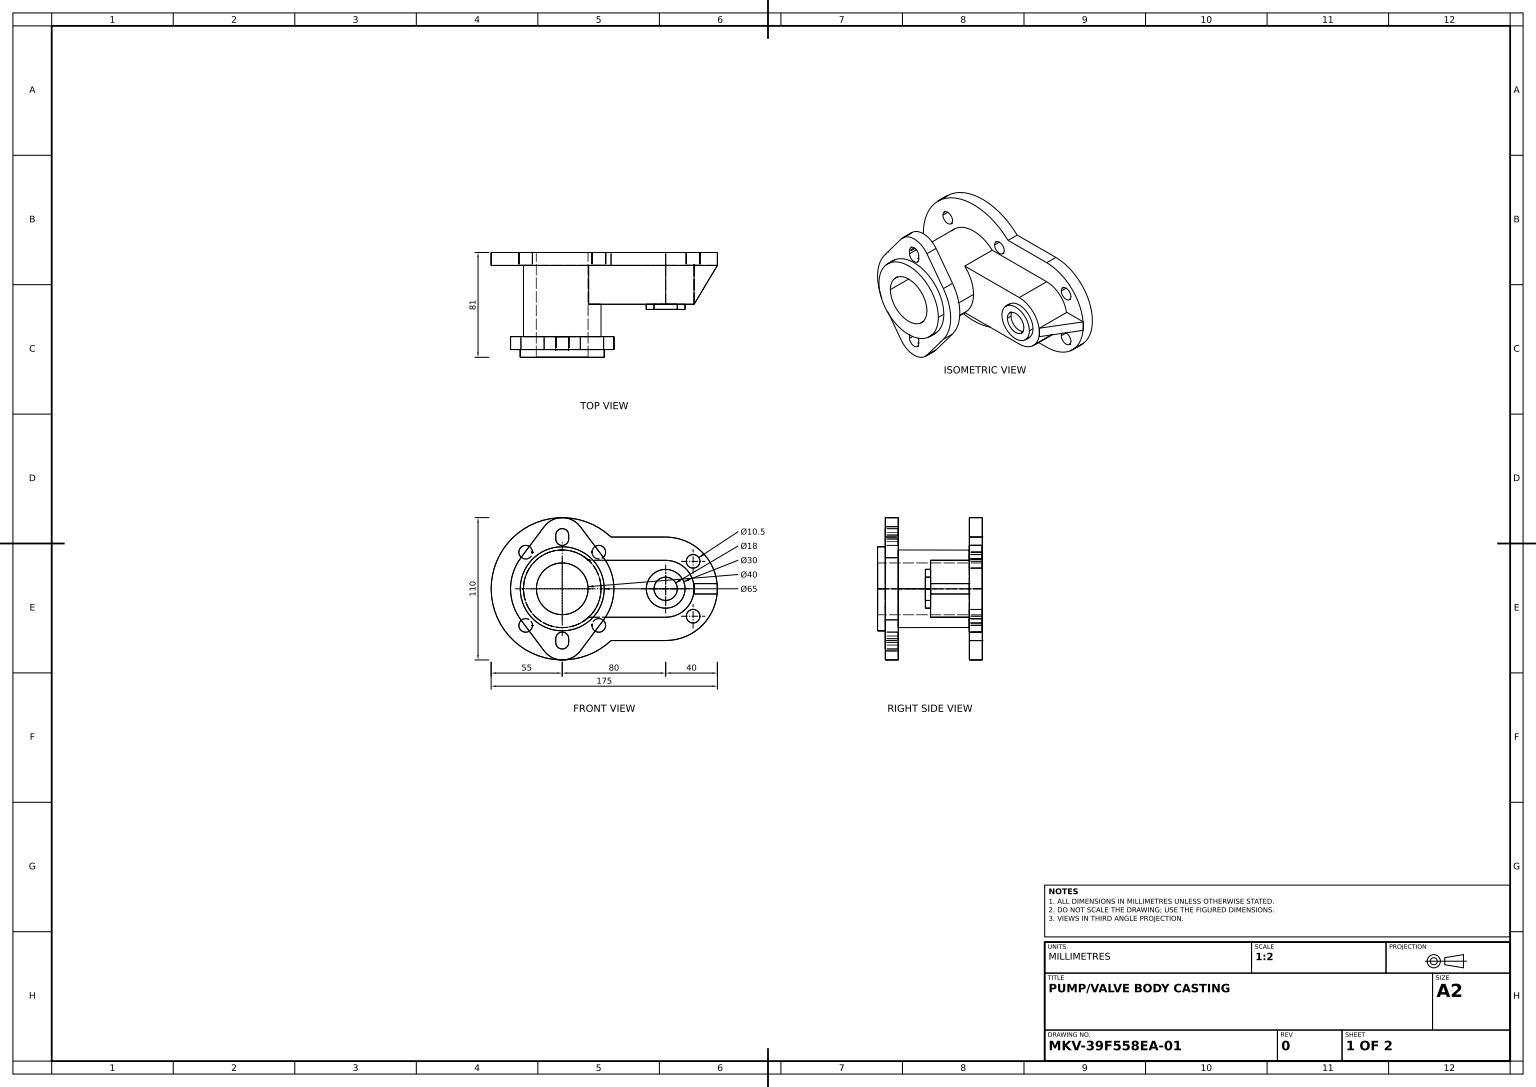
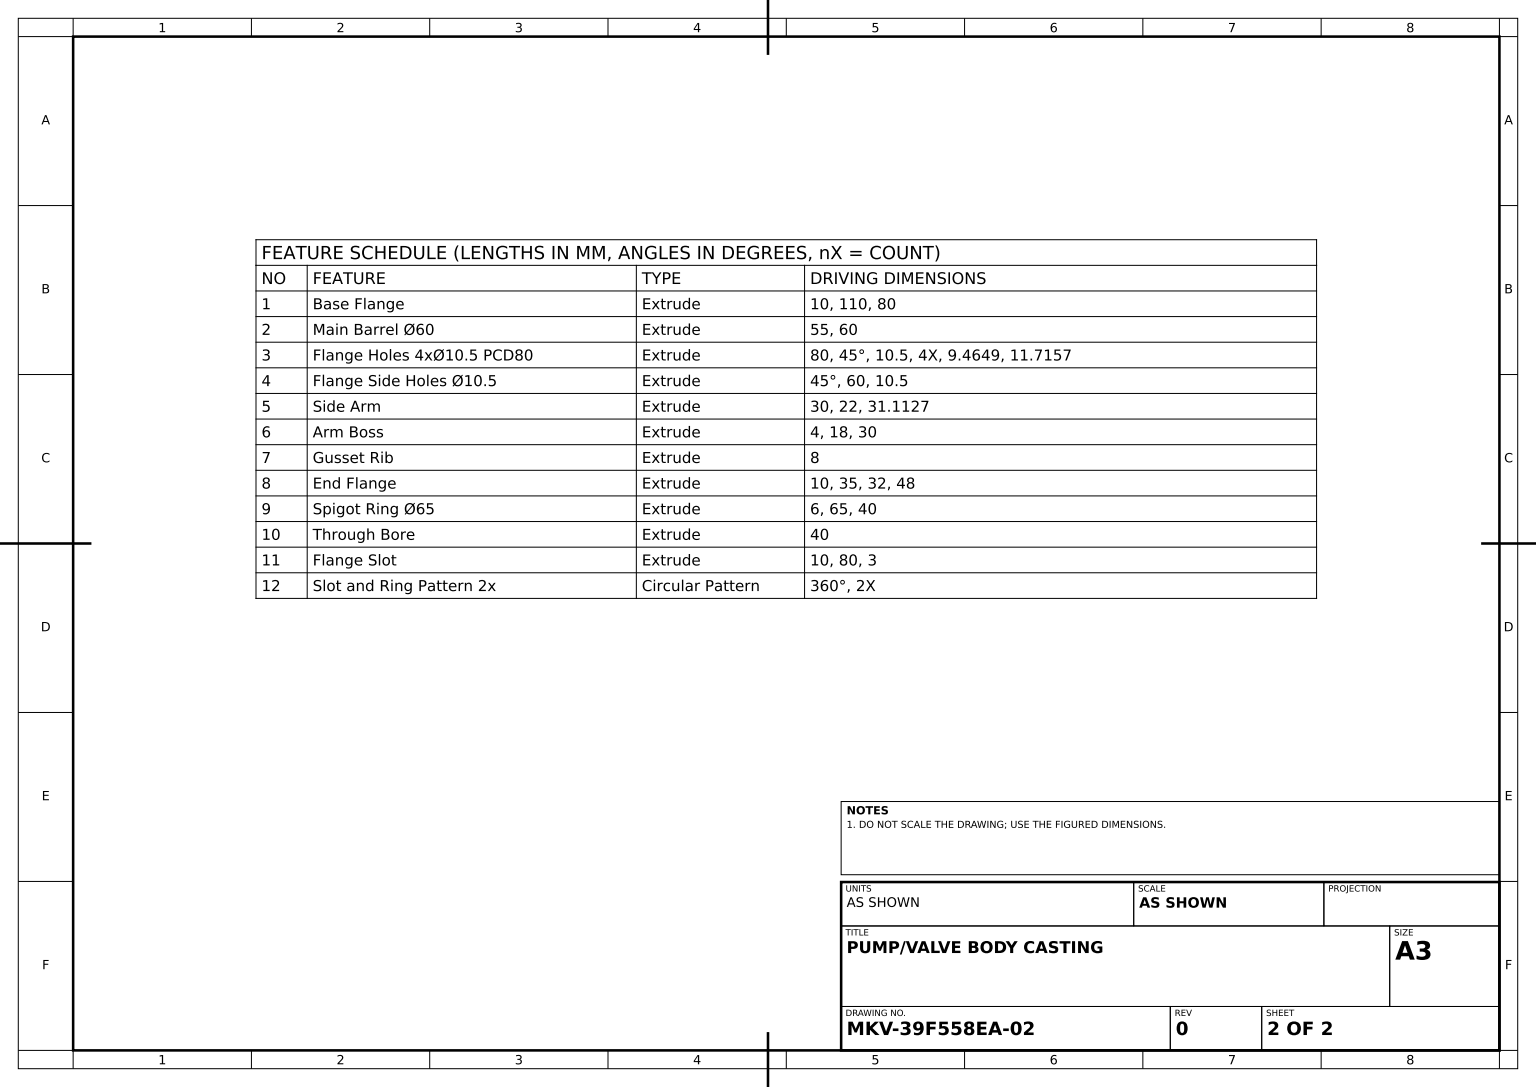
SolidWorks part; units mm, degrees
material "Plain Carbon Steel"
ref_plane "Front Plane" through (0, 0, 0) normal (0, 0, 1) x (1, 0, 0)
ref_plane "Top Plane" through (0, 0, 0) normal (0, 1, 0) x (1, 0, 0)
ref_plane "Right Plane" through (0, 0, 0) normal (1, 0, 0) x (0, 0, -1)
sketch "Base Flange Sketch" plane through (0, 0, 0) normal (0, 0, 1) x (1, 0, 0)
  line L0 (0, 0) -> (80, 0) construction
  line L1 (80, 40) -> (37.7492, 40)
  line L2 (80, -40) -> (37.7492, -40)
  arc A0 (37.7492, 40) -> (37.7492, -40) centre (0, 0) ccw
  arc A1 (80, -40) -> (80, 40) centre (80, 0) ccw
  dimension "D1" = 110
  dimension "D3" = 80
  dimension "D2" = 80
extrude "Base Flange" add sketch "Base Flange Sketch" along normal blind 10
sketch "Main Barrel Sketch" plane through (0, 0, 10) normal (0, 0, 1) x (1, 0, 0)
  circle A0 centre (0, 0) radius 30
  dimension "D1" = 60
extrude "Main Barrel Ø60" add sketch "Main Barrel Sketch" along normal blind 55
sketch "Flange Holes Sketch" plane through (0, 0, 10) normal (0, 0, 1) x (1, 0, 0)
  line L0 (80, 40) -> (37.7492, 40) construction
  line L2 (0, 0) -> (40, 0) construction
  line L3 (0, 0) -> (28.2843, 28.2843) construction
  circle A4 centre (0, 0) radius 40 construction
  circle A5 centre (28.2843, 28.2843) radius 5.25
  circle A6 centre (28.2843, -28.2843) radius 5.25
  circle A7 centre (-28.2843, -28.2843) radius 5.25
  circle A8 centre (-28.2843, 28.2843) radius 5.25
  dimension "D1" = 9.4649
  dimension "D2" = 80
  dimension "D4" = 10.5
  dimension "D3" = 45
  dimension "D6" = 11.7157
  dimension "D5" = 4
extrude "Flange Holes 4xØ10.5 PCD80" cut sketch "Flange Holes Sketch" against normal through all
sketch "Flange Side Holes Sketch" plane through (0, 0, 10) normal (0, 0, 1) x (1, 0, 0)
  line L0 (80, 0) -> (110, 0) construction
  line L1 (80, 0) -> (101.2132, 21.2132) construction
  line L2 (80, 0) -> (101.2132, -21.2132) construction
  circle A0 centre (80, 0) radius 30 construction
  circle A1 centre (101.2132, 21.2132) radius 5.25
  circle A2 centre (101.2132, -21.2132) radius 5.25
  dimension "D1" = 45
  dimension "D3" = 60
  dimension "D4" = 10.5
  dimension "D5" = 10.5
  dimension "D2" = 45
extrude "Flange Side Holes Ø10.5" cut sketch "Flange Side Holes Sketch" against normal through all
sketch "Side Arm Sketch" plane through (0, 0, 10) normal (0, 0, 1) x (1, 0, 0)
  line L0 (80, 22) -> (20.3961, 22)
  line L1 (80, -22) -> (20.3961, -22)
  arc A0 (80, -22) -> (80, 22) centre (80, 0) ccw
  circle A1 centre (0, 0) radius 30 construction
  circle A2 centre (0, 0) radius 30 construction
  arc A3 (20.3961, 22) -> (20.3961, -22) centre (-1.6039, 0) cw
  dimension "D1" = 22
  dimension "D2" = 31.1127
extrude "Side Arm" add sketch "Side Arm Sketch" along normal blind 30
sketch "Arm Boss Sketch" plane through (0, 0, 40) normal (0, 0, 1) x (1, 0, 0)
  circle A0 centre (80, 0) radius 15
  circle A1 centre (80, 0) radius 9
  dimension "D1" = 18
  dimension "D2" = 30
extrude "Arm Boss" add sketch "Arm Boss Sketch" along normal blind 4
ref_plane "Rib Plane" through (0, 0, 0) normal (0, 1, 0) x (1, 0, 0)
sketch "Gusset Rib Sketch" plane through (0, 0, 0) normal (0, 1, 0) x (1, 0, 0)
  line L0 (102, -40) -> (120, -10)
  line L1 (102, -40) -> (102, -10)
  line L2 (102, -10) -> (120, -10)
extrude "Gusset Rib" add sketch "Gusset Rib Sketch" along normal mid plane 8 separate body
sketch "End Flange Sketch" plane through (0, 0, 65) normal (0, 0, 1) x (1, 0, 0)
  line L0 (0, 0) -> (0, 55) construction
  line L1 (0, 0) -> (0, -55) construction
  line L2 (0, 55) -> (0, 37.5) construction
  line L3 (14, 48) -> (32, 24)
  line L4 (-14, 48) -> (-32, 24)
  line L5 (0, -55) -> (0, -37.5) construction
  line L6 (-14, -48) -> (-32, -24)
  line L7 (14, -48) -> (32, -24)
  arc A0 (-32, 24) -> (-32, -24) centre (0, 0) ccw
  arc A2 (37.7492, 40) -> (37.7492, -40) centre (0, 0) ccw construction
  arc A3 (14, 48) -> (-14, 48) centre (0, 37.5) ccw
  arc A5 (-14, -48) -> (14, -48) centre (0, -37.5) ccw
  arc A6 (32, -24) -> (32, 24) centre (0, 0) ccw
  dimension "D2" = 35
  dimension "D3" = 32
  dimension "D4" = 32
  dimension "D5" = 48
extrude "End Flange" add sketch "End Flange Sketch" along normal blind 10
sketch "Spigot Ring Sketch" plane through (0, 0, 75) normal (0, 0, 1) x (1, 0, 0)
  circle A0 centre (0, 0) radius 32.5
  circle A1 centre (0, 0) radius 20
  dimension "D1" = 65
  dimension "D2" = 40
extrude "Spigot Ring Ø65" add sketch "Spigot Ring Sketch" along normal blind 6
sketch "Through Bore Sketch" plane through (0, 0, 75) normal (0, 0, 1) x (1, 0, 0)
  circle A0 centre (0, 0) radius 20
  dimension "D1" = 40
extrude "Through Bore" cut sketch "Through Bore Sketch" against normal through all
sketch "Flange Slot Sketch" plane through (0, 0, 75) normal (0, 0, 1) x (1, 0, 0)
  line L0 (0, 0) -> (0, 40) construction
  line L1 (0, 0) -> (0, -40) construction
  line L2 (0, 38.5) -> (0, 41.5) construction
  line L3 (-5, 38.5) -> (-5, 41.5)
  line L4 (5, 38.5) -> (5, 41.5)
  circle A0 centre (0, 0) radius 40 construction
  arc A1 (-5, 38.5) -> (5, 38.5) centre (0, 38.5) ccw
  arc A2 (5, 41.5) -> (-5, 41.5) centre (0, 41.5) ccw
  point P7 (0, 40)
  dimension "D1" = 80
  dimension "D2" = 3
  dimension "D3" = 10
extrude "Flange Slot" cut sketch "Flange Slot Sketch" against normal blind 10
pattern_circular "Slot and Ring Pattern 2x" count 2 over 360 about axis through (0, 0, 0) along (0, 0, 1) of "Flange Slot"
